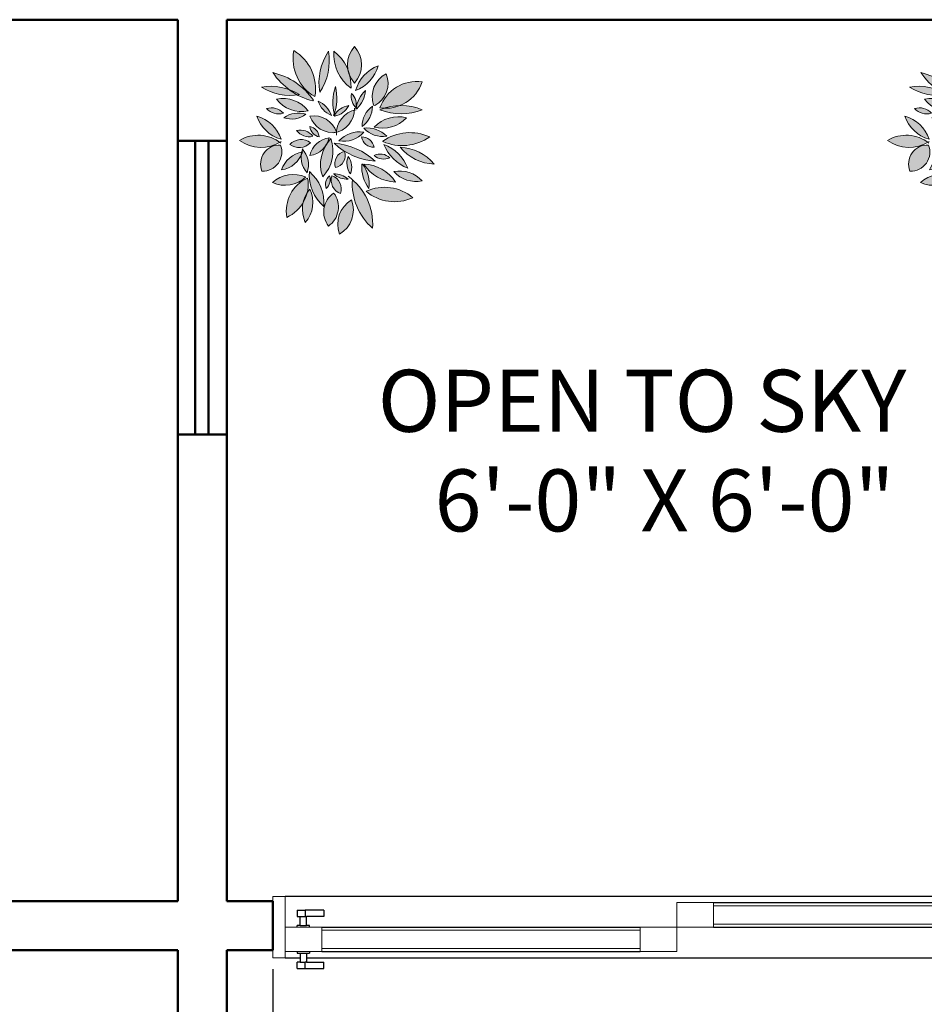
# Model space of a CAD drawing. Units: inches. Extents: x 64 to 1167, y 117 to 939.
# Tile 20 of 56: x 284 to 358, y 777 to 857. Entities that reach past the tile are written whole.
import ezdxf

# ---------------------------------------------------------------- set-up
doc = ezdxf.new("R2010")
doc.units = ezdxf.units.IN
doc.header["$MEASUREMENT"] = 0
for name, color, linetype, lineweight in [('A-ANNO-DIMS', 2, 'Continuous', 18), ('A-ANNO-TEXT', 7, 'Continuous', 25), ('A-DOOR', 4, 'Continuous', 25), ('A-FURN', 8, 'Continuous', 18), ('A-WALL', 7, 'Continuous', 50), ('cut', 6, 'Continuous', 18)]:
    doc.layers.add(name, color=color, linetype=linetype, lineweight=lineweight)
doc.styles.get("Standard").update_dxf_attribs({"font": 'arial.ttf'})
doc.dimstyles.get("Standard").update_dxf_attribs({"dimtxt": 0.18, "dimasz": 0.18, "dimexe": 0.18, "dimexo": 0.0625, "dimgap": 0.09, "dimtad": 0, "dimtih": 1, "dimtoh": 1, "dimdec": 4, "dimzin": 0, "dimdsep": 46, "dimtxsty": 'Standard', "dimcen": 0.09, "dimadec": 0, "dimazin": 0, "dimtfac": 1, "dimtdec": 4, "dimtofl": 0, "dimtmove": 0, "dimatfit": 3, "dimfxl": 1, "dimtolj": 1, "dimtzin": 0, "dimarcsym": 0})

# ---------------------------------------------------------------- blocks, each defined once
blk = doc.blocks.new('Sliding Glass Door pl')
for p, q in [((28.469, -0.005), (-35.531, -0.005)), ((-0.531, -0.505), (25.469, -0.505)), ((-34.531, -1.13), (-33.878, -1.13)), ((-34.531, -1.13), (-34.531, -1.63)), ((-33.878, -1.13), (-33.878, -1.63)), ((-32.355, -1.13), (-33.878, -1.13)), ((-32.355, -1.13), (-32.355, -1.63)), ((-34.531, -1.63), (-34.281, -1.63)), ((-34.281, -2.38), (-34.531, -2.38)), ((-34.531, -2.505), (-34.531, -2.38)), ((-34.281, -2.38), (-34.281, -1.63)), ((-34.281, -1.63), (-33.878, -1.63)), ((-34.281, -2.38), (-33.781, -2.38)), ((-33.878, -1.63), (-33.781, -1.63)), ((-33.781, -2.38), (-33.781, -1.63)), ((-32.355, -1.63), (-33.781, -1.63)), ((-33.531, -2.38), (-33.781, -2.38)), ((-33.531, -2.505), (-33.531, -2.38)), ((-32.531, -2.505), (-6.531, -2.505)), ((-0.531, -2.505), (25.469, -2.505)), ((-34.531, -4.505), (-34.531, -4.63)), ((-34.531, -4.63), (-34.281, -4.63)), ((-34.281, -4.63), (-33.781, -4.63)), ((-34.281, -4.63), (-34.281, -5.005)), ((-33.781, -4.63), (-33.781, -5.005)), ((-33.781, -4.63), (-33.531, -4.63)), ((-33.531, -4.505), (-33.531, -4.63)), ((-32.531, -4.505), (-6.531, -4.505)), ((-35.531, -5.005), (-34.281, -5.005)), ((-34.281, -5.38), (-34.531, -5.38)), ((-34.531, -5.88), (-34.531, -5.38)), ((-34.281, -5.005), (-34.281, -5.38)), ((-34.281, -5.38), (-33.878, -5.38)), ((-33.878, -5.88), (-33.878, -5.38)), ((-33.781, -5.38), (-33.878, -5.38)), ((-33.781, -5.005), (28.469, -5.005)), ((-33.781, -5.005), (-33.781, -5.38)), ((-33.781, -5.38), (-32.355, -5.38)), ((-32.355, -5.88), (-32.355, -5.38)), ((-34.531, -5.88), (-33.878, -5.88)), ((-33.878, -5.88), (-32.355, -5.88))]:
    blk.add_line(p, q)
at = {"layer": 'cut'}
for p, q in [((-36.531, -0.005), (-36.531, -5.005)), ((-35.531, -0.005), (-36.531, -0.005)), ((-35.531, -2.505), (-35.531, -0.005)), ((-0.531, -0.505), (-3.531, -0.505)), ((-3.531, -2.505), (-3.531, -0.505)), ((-0.531, -0.755), (-0.531, -0.505)), ((25.469, -0.755), (-0.531, -0.755)), ((-0.531, -2.255), (-0.531, -0.755)), ((28.469, -0.505), (25.469, -0.505)), ((25.469, -0.755), (25.469, -0.505)), ((25.469, -2.255), (25.469, -0.755)), ((29.469, -0.005), (28.469, -0.005)), ((28.469, -0.005), (28.469, -0.505)), ((28.469, -2.505), (28.469, -0.505)), ((29.469, -5.005), (29.469, -0.005)), ((25.469, -2.255), (-0.531, -2.255)), ((-0.531, -2.505), (-0.531, -2.255)), ((25.469, -2.505), (25.469, -2.255)), ((-34.531, -2.505), (-35.531, -2.505)), ((-35.531, -4.505), (-35.531, -2.505)), ((-34.531, -2.505), (-33.531, -2.505)), ((-32.531, -2.505), (-33.531, -2.505)), ((-32.531, -2.755), (-32.531, -2.505)), ((-6.531, -2.755), (-32.531, -2.755)), ((-32.531, -4.255), (-32.531, -2.755)), ((-3.531, -2.505), (-6.531, -2.505)), ((-6.531, -2.755), (-6.531, -2.505)), ((-6.531, -4.255), (-6.531, -2.755)), ((-3.531, -4.505), (-3.531, -2.505)), ((-0.531, -2.505), (-3.531, -2.505)), ((28.469, -2.505), (25.469, -2.505)), ((28.469, -2.505), (28.469, -5.005)), ((-35.531, -5.005), (-35.531, -4.505)), ((-34.531, -4.505), (-35.531, -4.505)), ((-33.531, -4.505), (-34.531, -4.505)), ((-32.531, -4.505), (-33.531, -4.505)), ((-6.531, -4.255), (-32.531, -4.255)), ((-32.531, -4.505), (-32.531, -4.255)), ((-6.531, -4.505), (-6.531, -4.255)), ((-3.531, -4.505), (-6.531, -4.505)), ((-36.531, -5.005), (-35.531, -5.005)), ((28.469, -5.005), (29.469, -5.005))]:
    blk.add_line(p, q, dxfattribs=at)
blk = doc.blocks.new('A$C172C5132')
at = {"linetype": 'ByBlock'}
h = blk.add_hatch(color=256, dxfattribs=at)
h.set_gradient(color1=(15, 138, 17), color2=(46, 92, 10), tint=1, name='HEMISPHERICAL')
h.paths.add_polyline_path([(0.08485, 0.04094, 0.236282), (0.10003, 0.00447, 0.236282)])
h.paths.add_polyline_path([(0.09513, 0.03216, 0.290628), (0.13031, 0.02738, 0.290628)])
h.paths.add_polyline_path([(0.07514, 0, 0.364082), (0.08427, 0.02564, 0.364082)])
h.paths.add_polyline_path([(0.0708, 0.03086, 0.428936), (0.06689, 0.00609, 0.428936)])
h.paths.add_polyline_path([(0.05256, 0.04694, 0.243055), (0.06342, 0.02086, 0.243055)])
h.paths.add_polyline_path([(0.05089, 0.03109, -0.075692), (0.04778, 0.02347, 0.164666), (0.04952, 0.00869, 0.298636), (0.05299, 0.0339, 0.03785)])
h.paths.add_polyline_path([(0.03562, 0.0126, 0.152567), (0.04778, 0.02347, -0.089408), (0.05089, 0.03109, 0.1023), (0.05125, 0.04216, 0.341288)])
h.paths.add_polyline_path([(0.02476, 0.03868, 0.299202), (0.04976, 0.04285, 0.299202)])
h.paths.add_polyline_path([(0.04745, 0.06366, 0.031182), (0.04682, 0.06163, -0.006707), (0.04735, 0.06172), (0.04735, 0.06172), (0.04735, 0.06172, -0.03138), (0.04644, 0.05941, 0.214704), (0.05082, 0.04607, 0.282795)])
h.paths.add_polyline_path([(0.06433, 0.06577, 0.211659), (0.06255, 0.04303, 0.281051), (0.06863, 0.07172, 0.038772), (0.06589, 0.06833, -0.044717)])
h.paths.add_polyline_path([(0.05299, 0.05911, 0.203733), (0.06433, 0.06577, -0.026656), (0.06589, 0.06833, 0.062829), (0.06727, 0.0723, 0.318582)])
h.paths.add_polyline_path([(0.0695, 0.0439, 0.403257), (0.07601, 0.03043, 0.403257)])
h.paths.add_polyline_path([(0.06515, 0.03434, 0.302607), (0.06776, 0.0439, 0.302607)])
h.paths.add_polyline_path([(0.0708, 0.0452, 0.20419), (0.08166, 0.04129, 0.20419)])
h.paths.add_polyline_path([(0.08166, 0.05824, 0.262138), (0.0834, 0.0452, 0.262138)])
h.paths.add_polyline_path([(0.0721, 0.04999, 0.44636), (0.07905, 0.06216, 0.44636)])
h.paths.add_polyline_path([(0.09339, 0.05259, 0.247085), (0.11728, 0.03912, 0.247085)])
h.paths.add_polyline_path([(0.07124, 0.06824, 0.171467), (0.10207, 0.05477, 0.171467)])
h.paths.add_polyline_path([(0.07471, 0.06998, 0.259278), (0.09339, 0.0765, 0.259278)])
h.paths.add_polyline_path([(0.09165, 0.07302, 0.365639), (0.10121, 0.0652, 0.365639)])
h.paths.add_polyline_path([(0.09339, 0.07954, 0.243415), (0.11076, 0.07346, 0.243415)])
h.paths.add_polyline_path([(0.10121, 0.05911, 0.307451), (0.11293, 0.05737, 0.307451)])
h.paths.add_polyline_path([(0.10859, 0.06737, 0.209633), (0.1264, 0.04955, 0.209633)])
h.paths.add_polyline_path([(0.12075, 0.0652, 0.21311), (0.14638, 0.05259, 0.21311)])
h.paths.add_polyline_path([(0.11597, 0.04694, 0.265719), (0.13726, 0.03999, 0.265719)])
h.paths.add_polyline_path([(0.10121, 0.08041, 0.271534), (0.12553, 0.08737, 0.271534)])
h.paths.add_polyline_path([(0.1204, 0.09653, -0.10541), (0.10842, 0.09449, 0.018052), (0.10555, 0.09345, 0.194763), (0.13726, 0.09345, 0.102488)])
h.paths.add_polyline_path([(0.10555, 0.09475, 0.024701), (0.10842, 0.09449, -0.072299), (0.1204, 0.09653, 0.220444), (0.13726, 0.11431, 0.361284)])
h.paths.add_polyline_path([(0.09208, 0.08085, 0.244188), (0.0999, 0.09606, 0.244188)])
h.paths.add_polyline_path([(0.08731, 0.10779, 0.236039), (0.10425, 0.12648, 0.236039)])
h.paths.add_polyline_path([(0.08427, 0.10562, 0.271887), (0.08751, 0.09507, 0.271887)])
h.paths.add_polyline_path([(0.07295, 0.07656, -0.001193), (0.07298, 0.07648, 0.325344), (0.08635, 0.09313, 0.324468)])
h.paths.add_polyline_path([(0.07129, 0.09046, 0.143951), (0.0721, 0.11084, 0.143951)])
h.paths.add_polyline_path([(0.05907, 0.09997, 0.207976), (0.06906, 0.0891, 0.207976)])
h.paths.add_polyline_path([(0.06038, 0.10649, 0.190107), (0.06689, 0.13735, 0.190107)])
h.paths.add_polyline_path([(0.0708, 0.13735, 0.252904), (0.08383, 0.10953, 0.067921), (0.08315, 0.11824, -0.074796), (0.08133, 0.12397, 0.134159)])
h.paths.add_polyline_path([(0.08133, 0.12397, -0.046564), (0.08315, 0.11824, 0.072445), (0.08644, 0.11344, 0.391074), (0.08644, 0.14083, 0.229731)])
h = blk.add_hatch(color=256, dxfattribs=at)
h.set_gradient(color1=(12, 110, 14), color2=(39, 78, 9), tint=1, name='HEMISPHERICAL')
h.paths.add_polyline_path([(0.0278, 0.10127, 0.287265), (0.05169, 0.09258, 0.287265)])
h.paths.add_polyline_path([(0.03345, 0.08737, 0.245454), (0.04995, 0.08997, 0.245454)])
h.paths.add_polyline_path([(0.05299, 0.08867, 0.362884), (0.07295, 0.0765, -0.000877), (0.07295, 0.07656, 0.362272)])
h.paths.add_polyline_path([(0.05299, 0.08085, 0.33327), (0.05994, 0.07302, 0.33327)])
h.paths.add_polyline_path([(0.043, 0.0778, 0.302945), (0.05516, 0.07346, 0.302945)])
h.paths.add_polyline_path([(0.03779, 0.06737, 0.378763), (0.05343, 0.06868, 0.378763)])
h.paths.add_polyline_path([(0.03171, 0.04825, 0.247698), (0.04644, 0.05941, -0.032946), (0.04682, 0.06163, 0.274039)])
h.paths.add_polyline_path([(0.01694, 0.04738, 0.549808), (0.03084, 0.06694, 0.549808)])
h.paths.add_polyline_path([(0, 0.07041, 0.297781), (0.03041, 0.06901, 0.297781)])
h.paths.add_polyline_path([(0.01303, 0.08867, 0.248111), (0.03127, 0.07128, 0.248111)])
h.paths.add_polyline_path([(0.02041, 0.09432, 0.290415), (0.03301, 0.09084, 0.290415)])
h.paths.add_polyline_path([(0.01651, 0.1104, 0.175406), (0.04366, 0.10452, -0.037323), (0.03721, 0.10862, 0.129374)])
h.paths.add_polyline_path([(0.02519, 0.12127, 0.085647), (0.03721, 0.10862, -0.054384), (0.04517, 0.10475), (0.04517, 0.10475, -0.009351), (0.04366, 0.10452, 0.060507), (0.0552, 0.10004), (0.05561, 0.10063, 0.185254)])
h.paths.add_polyline_path([(0.04083, 0.13779, 0.313266), (0.05659, 0.10326), (0.05673, 0.10333, 0.313266)])
h.paths.add_polyline_path([(0.07124, 0.0891), (0.07156, 0.08865, 0.230232), (0.08209, 0.09649, 0.230232)])
h.paths.add_polyline_path([(0.08774, 0.09432), (0.08812, 0.09413, 0.179345), (0.09469, 0.10779, 0.179345)])
h.paths.add_polyline_path([(0.10078, 0.09682), (0.10164, 0.09649, 0.378282), (0.11033, 0.1204, 0.378282)])
h = blk.add_hatch(color=256, dxfattribs=at)
h.set_gradient(color1=(12, 110, 14), color2=(39, 78, 9), tint=1, name='HEMISPHERICAL')
h.paths.add_polyline_path([(0.10769, 0.0699), (0.10772, 0.06954, 0.262244), (0.1429, 0.07302, 0.262244)])
h = blk.add_hatch(color=256)
h.set_gradient(color1=(12, 110, 14), color2=(39, 78, 9), tint=1, name='HEMISPHERICAL')
h.paths.add_polyline_path([(0.09252, 0.05259), (0.092, 0.05245, 0.192472), (0.0973, 0.03434, 0.192472)])
for p, q in [((0.0552, 0.10004), (0.05561, 0.10063)), ((0.05659, 0.10326), (0.05673, 0.10333)), ((0.10164, 0.09649), (0.10078, 0.09682)), ((0.07156, 0.08865), (0.07124, 0.0891)), ((0.08812, 0.09413), (0.08774, 0.09432)), ((0.10772, 0.06954), (0.10769, 0.0699)), ((0.09252, 0.05259), (0.092, 0.05245))]:
    blk.add_line(p, q, dxfattribs=at)
for centre, radius, start, end in [((0.10127, 0.12714), 0.02018, 137.28165, 222.71835), ((0.07161, 0.12714), 0.02018, 317.28165, 42.71835), ((0.07355, 0.13186), 0.03326, 169.7437, 239.31975), ((0.02398, 0.10911), 0.03326, 349.97973, 59.55579), ((0.10275, 0.11366), 0.04298, 146.55062, 189.60629), ((0.02452, 0.13018), 0.04298, 326.55062, 9.60629), ((0.10306, 0.1355), 0.03231, 176.7146, 233.4855), ((0.05158, 0.11138), 0.03231, 356.7146, 53.4855), ((0.11447, 0.1002), 0.02821, 111.24988, 164.37382), ((0.07708, 0.13408), 0.02821, 291.24988, 344.37382), ((0.01351, 0.07132), 0.0513, 34.85184, 76.83294), ((0.06785, 0.14976), 0.0513, 213.73456, 255.71565), ((0.1189, 0.1032), 0.01922, 116.50487, 199.38784), ((0.09245, 0.11337), 0.01922, 298.58777, 21.47073), ((0.02347, 0.07018), 0.04082, 57.8807, 99.81892), ((0.13317, 0.08546), 0.02915, 81.94051, 161.39642), ((0.10964, 0.12361), 0.02915, 261.94051, 341.39642), ((0.03821, 0.14498), 0.04082, 237.8807, 279.81892), ((0.10635, 0.09926), 0.03615, 161.32788, 196.37849), ((0.03704, 0.10203), 0.03615, 339.04336, 14.09398), ((0.09488, 0.10311), 0.0109, 166.67124, 231.57876), ((0.0769, 0.09758), 0.0109, 342.60507, 47.51259), ((0.10939, 0.09168), 0.02181, 132.38089, 173.05133), ((0.07297, 0.10982), 0.02181, 313.98943, 354.65987), ((0.0328, 0.07785), 0.02395, 37.94947, 102.05959), ((0.04669, 0.116), 0.02395, 217.94947, 282.05959), ((0.05157, 0.08305), 0.01851, 19.09754, 66.09222), ((0.07657, 0.10603), 0.01851, 199.09754, 246.09222), ((0.08426, 0.08163), 0.01502, 98.30282, 150.16438), ((0.06876, 0.1034), 0.01502, 280.74042, 332.60199), ((0.1214, 0.05429), 0.04225, 67.9577, 112.0423), ((0.02397, 0.08265), 0.0122, 42.17982, 106.95612), ((0.02945, 0.10251), 0.0122, 222.17982, 286.95612), ((0.04419, 0.07287), 0.01805, 71.39699, 126.56013), ((0.0392, 0.10447), 0.01805, 251.39699, 306.56013), ((0.05571, 0.07065), 0.01823, 18.72648, 98.58194), ((0.06822, 0.09399), 0.01815, 278.32555, 1.78158), ((0.09108, 0.07561), 0.01815, 100.59637, 184.05239), ((0.08135, 0.09598), 0.01856, 305.35468, 0.24439), ((0.11064, 0.08092), 0.01856, 125.35468, 180.24439), ((0.1214, 0.13261), 0.04225, 247.9577, 292.0423), ((0.03859, 0.09723), 0.02696, 198.50932, 254.2466), ((0.00571, 0.06273), 0.02696, 18.50932, 74.2466), ((0.07025, 0.09452), 0.01823, 198.72648, 278.58194), ((0.1193, 0.06314), 0.02501, 75.5726, 136.33853), ((0.10744, 0.10463), 0.02501, 255.5726, 316.33853), ((0.01413, 0.04645), 0.02782, 52.09547, 120.52382), ((0.04583, 0.06651), 0.01164, 36.62615, 104.04181), ((0.05234, 0.08475), 0.01164, 216.62615, 284.04181), ((0.05125, 0.0723), 0.00872, 4.751, 78.47786), ((0.06168, 0.08157), 0.00872, 184.751, 258.47786), ((0.08991, 0.05644), 0.02036, 80.1717, 138.31359), ((0.07819, 0.09004), 0.02036, 260.1717, 318.31359), ((0.0962, 0.05971), 0.02003, 43.3367, 98.0592), ((0.10795, 0.09329), 0.02003, 223.3367, 278.0592), ((0.12806, 0.0402), 0.03602, 65.66929, 124.4476), ((0.01628, 0.09298), 0.02782, 234.19362, 302.62197), ((0.0301, 0.05275), 0.01421, 86.99646, 202.20578), ((0.01768, 0.06157), 0.01421, 266.99646, 22.20578), ((0.04635, 0.05918), 0.01184, 53.27719, 136.25647), ((0.04487, 0.07686), 0.01184, 233.27719, 316.25647), ((0.05083, 0.07577), 0.0168, 277.38832, 349.07027), ((0.06943, 0.05564), 0.0168, 96.3902, 168.07215), ((0.08909, 0.05239), 0.02815, 136.63556, 199.4278), ((0.04209, 0.06236), 0.02815, 316.63556, 19.4278), ((0.10572, 0.10515), 0.05051, 226.93945, 265.85826), ((0.06759, 0.01786), 0.05051, 46.93945, 85.85826), ((0.09179, 0.06345), 0.00957, 10.523, 90.86046), ((0.10106, 0.07477), 0.00957, 190.523, 270.86046), ((0.12223, 0.10252), 0.03602, 246.25516, 305.03347), ((0.09718, 0.03816), 0.03137, 21.30152, 68.66), ((0.13781, 0.07877), 0.03137, 201.30152, 248.66), ((0.0285, 0.06778), 0.0198, 279.33237, 342.1699), ((0.05056, 0.04218), 0.0198, 99.33237, 162.1699), ((0.06344, 0.05761), 0.0171, 157.71225, 222.42351), ((0.03483, 0.05213), 0.0171, 339.26102, 43.97228), ((0.08104, 0.05295), 0.00941, 102.16354, 198.37984), ((0.07012, 0.05919), 0.00941, 282.16354, 18.37984), ((0.10579, 0.04961), 0.01055, 47.38732, 115.74759), ((0.11945, 0.0302), 0.03502, 39.74877, 87.87017), ((0.14768, 0.08759), 0.03502, 219.74877, 267.87017), ((0.09411, 0.05327), 0.01341, 158.21186, 216.96735), ((0.07095, 0.05018), 0.01341, 338.21186, 36.96735), ((0.11731, 0.05001), 0.02542, 174.4977, 218.07611), ((0.07207, 0.03749), 0.02542, 352.87776, 36.45617), ((0.11813, 0.06855), 0.02945, 212.81844, 268.33426), ((0.09253, 0.02316), 0.02945, 32.81844, 88.33426), ((0.10835, 0.06688), 0.01055, 227.38732, 295.74759), ((0.04043, 0.02175), 0.02307, 65.48932, 132.77516), ((0.08323, 0.04441), 0.03077, 175.28394, 229.92847), ((0.03275, 0.02339), 0.03077, 355.28394, 49.92847), ((0.07164, 0.03051), 0.01472, 47.10765, 93.27006), ((0.08082, 0.05599), 0.01472, 227.10765, 273.27006), ((0.12054, 0.02485), 0.02255, 42.14373, 101.66666), ((0.1327, 0.06208), 0.02255, 222.14373, 281.66666), ((0.03409, 0.05979), 0.02307, 246.14593, 313.43178), ((0.06256, 0.01726), 0.02735, 114.43033, 189.80696), ((0.02431, 0.0375), 0.02735, 294.43033, 9.80696), ((0.07363, 0.03716), 0.00894, 131.08234, 198.42695), ((0.05928, 0.04107), 0.00894, 311.08234, 18.42695), ((0.07975, 0.04055), 0.01079, 161.8817, 249.73011), ((0.06576, 0.03378), 0.01079, 341.8817, 69.73011), ((0.056, 0.00754), 0.04414, 356.00956, 54.57675), ((0.12888, 0.03787), 0.04414, 176.00956, 229.18601), ((0.07048, 0.01865), 0.0232, 138.89686, 205.40693), ((0.03203, 0.02395), 0.0232, 318.89686, 25.40693), ((0.08063, 0.01661), 0.01731, 124.60082, 217.46578), ((0.05706, 0.02033), 0.01731, 304.60082, 37.46578), ((0.10895, 0.00207), 0.03312, 49.85059, 114.67195), ((0.11648, 0.05748), 0.03312, 229.85059, 294.67195), ((0.09498, 0.00739), 0.02117, 120.40857, 200.43118), ((0.06443, 0.01826), 0.02117, 300.40857, 20.43118)]:
    blk.add_arc(centre, radius, start, end, dxfattribs=at)
blk = doc.blocks.new('*D94')
at = {"layer": 'A-ANNO-DIMS', "color": 0, "lineweight": -2, "transparency": 16777216}
for p, q in [((304.86, 779.638), (304.86, 769.621)), ((370.86, 779.638), (370.86, 769.621)), ((305.04, 769.801), (336.237, 769.801)), ((370.68, 769.801), (339.483, 769.801))]:
    blk.add_line(p, q, dxfattribs=at)
for points in [[(305.04, 769.831), (305.04, 769.771), (304.86, 769.801)], [(370.68, 769.831), (370.68, 769.771), (370.86, 769.801)]]:
    blk.add_solid(points, dxfattribs=at)
at = {"layer": 'Defpoints', "color": 0, "lineweight": -2, "transparency": 16777216}
for p in [(304.86, 779.701), (370.86, 779.701), (370.86, 769.801)]:
    blk.add_point(p, dxfattribs=at)
at = {"layer": 'A-ANNO-DIMS', "color": 0, "transparency": 16777216, "insert": (337.86, 769.801), "char_height": 0.18, "attachment_point": 5}
blk.add_mtext('\\A1;SLIDING GLASS DOOR 66', dxfattribs=at)

msp = doc.modelspace()

# ---------------------------------------------------------------- linework, layer by layer
at = {"layer": 'A-WALL'}
for p, q in [((297.107, 857.2), (183.107, 857.2)), ((297.107, 857.2), (297.107, 785.2)), ((301.107, 857.2), (301.107, 785.2)), ((373.107, 857.2), (301.107, 857.2)), ((297.107, 847.311), (301.107, 847.311)), ((298.524, 847.311), (298.524, 823.311)), ((299.595, 847.311), (299.595, 823.311)), ((297.107, 823.311), (301.107, 823.311)), ((297.107, 785.2), (183.107, 785.2)), ((304.86, 785.2), (301.107, 785.2)), ((304.86, 785.2), (304.86, 781.2)), ((297.107, 781.2), (166.795, 781.2)), ((297.107, 781.2), (297.107, 637.2)), ((301.107, 781.2), (301.107, 637.2)), ((304.86, 781.2), (301.107, 781.2))]:
    msp.add_line(p, q, dxfattribs=at)

# ---------------------------------------------------------------- block references
at = {"layer": 'A-DOOR'}
msp.add_blockref('Sliding Glass Door pl', (341.391, 785.581), dxfattribs=at)
at = {"layer": 'A-FURN', "xscale": 108.7946212322529, "yscale": 108.7946212322529, "zscale": 108.7946212322529}
for p in [(302.131, 839.681), (355.073, 839.681)]:
    msp.add_blockref('A$C172C5132', p, dxfattribs=at)

# ---------------------------------------------------------------- texts
at = {"layer": 'A-ANNO-TEXT'}
for s, p in [('OPEN TO SKY', (313.435, 823.536)), ('   6\'-0" X 6\'-0"', (313.435, 815.4))]:
    msp.add_text(s, height=5.06489, dxfattribs=at).set_placement(p)

# ---------------------------------------------------------------- dimensions: what is measured, and where the dimension line sits
at = {"layer": 'A-ANNO-DIMS'}
dim = msp.add_linear_dim(base=(370.86, 769.801), p1=(304.86, 779.701), p2=(370.86, 779.701), text='SLIDING GLASS DOOR <>', dimstyle='Standard', override={"dimdec": 0, "dimlfac": 1, "dimrnd": 0, "dimzin": 0, "dimdsep": 46, "dimlunit": 2}, dxfattribs=at)
dim.commit()
dim.dimension.update_dxf_attribs({"geometry": '*D94', "text_midpoint": (337.86, 769.801)})

doc.saveas('drawing.dxf')
